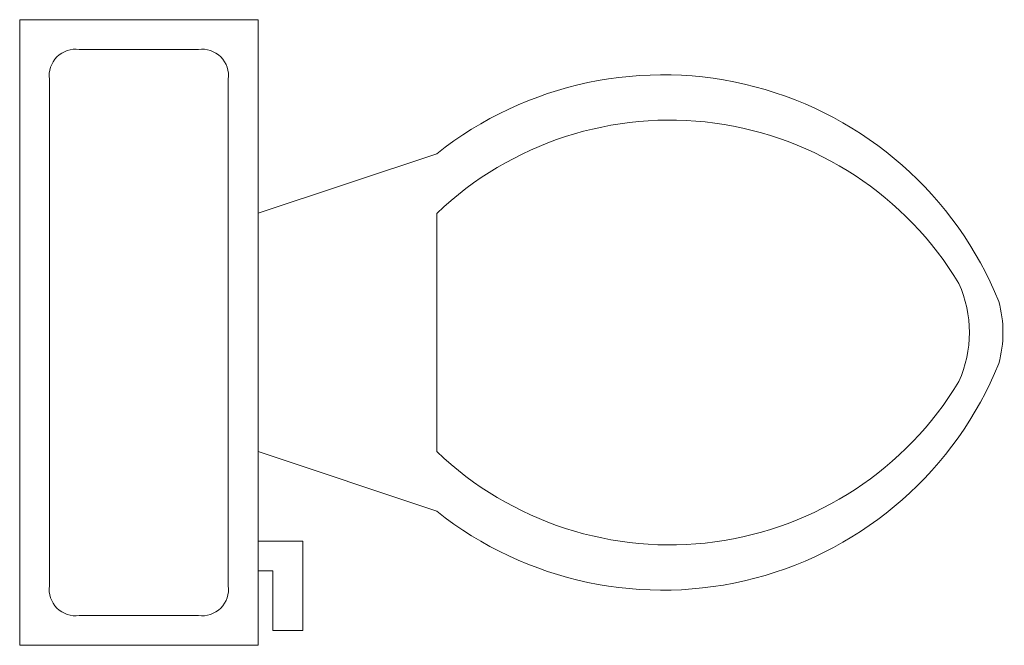
# Model space of a CAD drawing. Units: inches. Extents: x 1885 to 4781, y 1153 to 4395.
# Tile 7 of 7: x 4748 to 4781, y 4374 to 4395. Entities that reach past the tile are written whole.
import ezdxf

# ---------------------------------------------------------------- set-up
doc = ezdxf.new("R2010")
doc.units = ezdxf.units.IN
doc.layers.add('A-FLOR-FIXT', color=11, linetype='Continuous', lineweight=18, true_color=0xf27172)

# ---------------------------------------------------------------- blocks, each defined once
blk = doc.blocks.new('Toilet - top')
for p, q in [((9.5, -6), (9.5, -2)), ((-8, -8.5), (-8, -8)), ((-7, -8), (-7, -9.5)), ((-4, -8), (-6, -14)), ((4, -8), (6, -14)), ((-10, -8.5), (-8, -8.5)), ((-10, -9.5), (-10, -8.5)), ((-7, -9.5), (-10, -9.5)), ((4, -14), (-4, -14))]:
    blk.add_line(p, q)
blk.add_lwpolyline([(10.5, -8), (10.5, 0), (-10.5, 0), (-10.5, -8)], close=True)
for points in [[(8.5, -1), (-8.5, -1)], [(-9.5, -2), (-9.5, -6)], [(-8.5, -7), (8.5, -7)]]:
    blk.add_lwpolyline(points)
for centre, radius, start, end in [((-8.625, -1.875), 0.884, 81.8699, 188.1301), ((8.625, -1.875), 0.884, 351.8699, 98.1301), ((-8.625, -6.125), 0.884, 171.8699, 278.1301), ((8.625, -6.125), 0.884, 261.8699, 8.1301), ((3.52, -21.58), 12.169, 141.4691, 247.9714), ((4.2, -21.817), 11.329, 136.3677, 238.9468), ((-3.519, -21.58), 12.169, 292.0284, 38.5307), ((-4.2, -21.817), 11.329, 301.053, 43.6321), ((0, -27.876), 4, 245.7318, 294.2682), ((0, -29), 4, 254.8605, 285.1395)]:
    blk.add_arc(centre, radius, start, end)

msp = doc.modelspace()

# ---------------------------------------------------------------- block references
at = {"layer": 'A-FLOR-FIXT', "rotation": 90}
msp.add_blockref('Toilet - top', (4747.865, 4384.504), dxfattribs=at)

doc.saveas('drawing.dxf')
